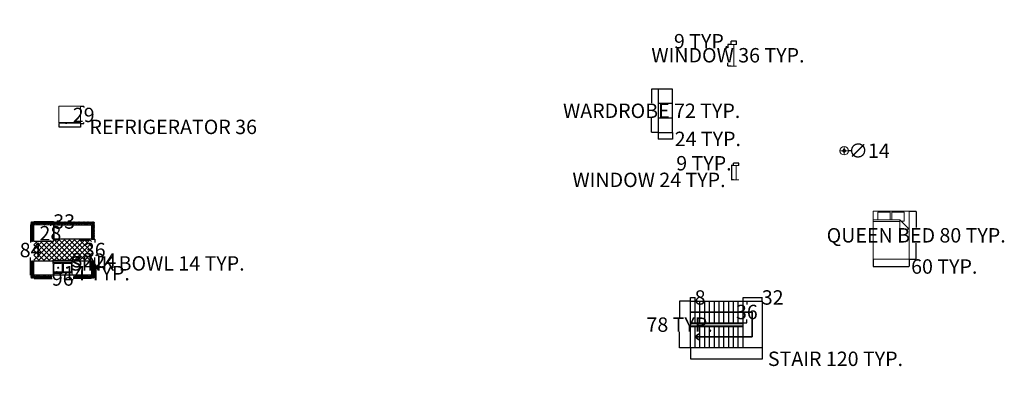
# Model space of a CAD drawing. Units: inches. Extents: x -1226 to 4538, y -998 to 1029.
# Tile 5 of 5: x 2895 to 4538, y 408 to 1029. Entities that reach past the tile are written whole.
import ezdxf

# ---------------------------------------------------------------- set-up
doc = ezdxf.new("R2010")
doc.units = ezdxf.units.IN
doc.header["$MEASUREMENT"] = 0
for name, color, linetype, lineweight in [('A-ANNO-DIMS', 2, 'Continuous', 18), ('A-ANNO-SYMB', 7, 'Continuous', 35), ('A-EQPM', 8, 'Continuous', 18), ('A-FLOR-CASE', 8, 'Continuous', 25), ('A-FLOR-FIXT', 9, 'Continuous', 18), ('A-FLOR-PATT', 2, 'Continuous', 13), ('A-FLOR-STRS', 7, 'Continuous', 25), ('A-FURN', 8, 'Continuous', 18), ('A-GLAZ', 3, 'Continuous', 18), ('A-WALL-PATT', 1, 'Continuous', 13)]:
    doc.layers.add(name, color=color, linetype=linetype, lineweight=lineweight)
doc.styles.get("Standard").update_dxf_attribs({"font": 'arial.ttf'})
doc.dimstyles.get("Standard").update_dxf_attribs({"dimtxt": 24, "dimasz": 0.18, "dimexe": 0.18, "dimexo": 0.0625, "dimgap": 0.09, "dimtad": 0, "dimtih": 1, "dimtoh": 1, "dimdec": 0, "dimzin": 0, "dimdsep": 46, "dimlunit": 4, "dimtxsty": 'Standard', "dimcen": 0.09, "dimadec": 0, "dimazin": 0, "dimtfac": 1, "dimtdec": 0, "dimtofl": 0, "dimtmove": 0, "dimatfit": 3, "dimfxl": 1, "dimtolj": 1, "dimtzin": 0, "dimarcsym": 0})

# ---------------------------------------------------------------- blocks, each defined once
blk = doc.blocks.new('Bed - Queen')
for p, q in [((0, -80.00003), (0, 0)), ((0, 0), (59.99999, 0)), ((59.99999, 0), (59.99999, -80.00003)), ((0, -14.4), (44.8, -14.4)), ((7.99999, -1.2), (28.79998, -1.2)), ((7.99999, -14.4), (7.99999, -1.2)), ((28.79998, -1.2), (28.79998, -14.4)), ((31.19999, -1.2), (51.99999, -1.2)), ((31.19999, -14.4), (31.19999, -1.2)), ((59.99999, -29.6), (44.8, -14.4)), ((44.8, -14.4), (44.8, -29.6)), ((51.99999, -16.4), (46.79936, -16.4)), ((51.99999, -1.2), (51.99999, -16.4)), ((44.8, -16.8), (0, -16.8)), ((44.8, -29.6), (59.99999, -29.6)), ((59.99999, -80.00003), (0, -80.00003))]:
    blk.add_line(p, q)
blk = doc.blocks.new('Lamp - Table')
for p, q in [((-1, 0), (-7, 0)), ((0, 3), (-3, 0)), ((-3, 0), (0, -3)), ((0, 7), (0, 1)), ((3, 0), (0, 3)), ((0, -3), (3, 0)), ((1, 0), (7, 0)), ((0, -1), (0, -7))]:
    blk.add_line(p, q)
for radius in [7, 1]:
    blk.add_circle((0, 0), radius)
blk = doc.blocks.new('Refrigerator-2 door - 36 in top')
for p, q in [((0, -26.999999), (36, -26.999999)), ((11, -27.999999), (11, -28.999999)), ((11, -28.999999), (13, -28.999999)), ((12, -26.999999), (12, -28.999999)), ((13, -28.999999), (13, -27.999999))]:
    blk.add_line(p, q)
blk.add_lwpolyline([(0, -27.999999), (0, 0), (36, 0), (36, -27.999999)], close=True)
blk = doc.blocks.new('WIN-36')
for p, q in [((0, 36), (9, 36)), ((4.5, 0), (4.5, 36)), ((0, 0), (9, 0))]:
    blk.add_line(p, q)
blk = doc.blocks.new('WIN-24')
for p, q in [((0, 24), (9, 24)), ((4.5, 0), (4.5, 24)), ((0, 0), (9, 0))]:
    blk.add_line(p, q)
blk = doc.blocks.new('WARDROBE-72X24')
for p, q in [((72, 24), (0, 24)), ((0, 24), (0, 0)), ((24, 24), (24, 0)), ((48, 24), (48, 0)), ((72, 0), (72, 24)), ((0, 0), (72, 0))]:
    blk.add_line(p, q)
blk = doc.blocks.new('STAIR-RETURN-120X78')
for p, q in [((0, 0), (0, 120)), ((0, 120), (78, 120)), ((78, 120), (78, 0)), ((42, 88), (0, 88)), ((36, 0), (36, 88)), ((37, 0), (37, 88)), ((41, 0), (41, 88)), ((42, 0), (42, 88)), ((78, 88), (42, 88)), ((36, 80), (0, 80)), ((36, 72), (0, 72)), ((78, 80), (42, 80)), ((78, 72), (42, 72)), ((36, 64), (0, 64)), ((36, 56), (0, 56)), ((78, 64), (42, 64)), ((78, 56), (42, 56)), ((36, 48), (0, 48)), ((36, 40), (0, 40)), ((78, 48), (42, 48)), ((78, 40), (42, 40)), ((36, 32), (0, 32)), ((36, 24), (0, 24)), ((78, 32), (42, 32)), ((78, 24), (42, 24)), ((36, 16), (0, 16)), ((36, 8), (0, 8)), ((78, 16), (42, 16)), ((78, 8), (42, 8)), ((37, 0), (0, 0)), ((78, 0), (41, 0))]:
    blk.add_line(p, q)
blk = doc.blocks.new('STAIR-DIRECTION-RETURN')
for p, q in [((0, 0), (0, 103.3)), ((0, 103.3), (40.8, 103.3)), ((40.8, 103.3), (40.8, 8)), ((40.8, 8), (35.9, 13.9)), ((40.8, 8), (45.7, 13.9))]:
    blk.add_line(p, q)
blk = doc.blocks.new('SINK-BOWL-COMPACT')
blk.add_line((13.8, 1), (13.8, 13))
for points in [[(0, 1), (0, 13)], [(1, 14), (12.8, 14)], [(12.8, 0), (1, 0)]]:
    blk.add_lwpolyline(points)
for radius in [1, 0.5]:
    blk.add_circle((7, 7), radius)
for centre, start, end in [((1, 13), 90, 180), ((1, 1), 180, 270), ((12.8, 13), 0, 90), ((12.8, 1), 270, 0)]:
    blk.add_arc(centre, 1, start, end)
blk = doc.blocks.new('*D22')
at = {"layer": 'A-ANNO-DIMS', "color": 0, "lineweight": -2, "transparency": 16777216}
for p, q in [((4082.1, 987.5), (4076.5, 987.5)), ((4076.7, 987.4), (4076.7, 982.1)), ((4076.7, 951.7), (4076.7, 957)), ((4082.1, 951.5), (4076.5, 951.5))]:
    blk.add_line(p, q, dxfattribs=at)
at = {"layer": 'A-ANNO-DIMS', "color": 0, "transparency": 16777216}
for points in [[(4076.7, 987.4), (4076.8, 987.4), (4076.7, 987.5)], [(4076.7, 951.7), (4076.8, 951.7), (4076.7, 951.5)]]:
    blk.add_solid(points, dxfattribs=at)
at = {"layer": 'Defpoints', "color": 0, "transparency": 16777216}
for p in [(4082.1, 987.5), (4076.7, 951.5), (4082.1, 951.5)]:
    blk.add_point(p, dxfattribs=at)
at = {"layer": 'A-ANNO-DIMS', "color": 0, "transparency": 16777216, "insert": (4076.7, 969.5), "char_height": 24, "attachment_point": 5}
blk.add_mtext('\\A1;WINDOW 36 TYP.', dxfattribs=at)
blk = doc.blocks.new('*D23')
at = {"layer": 'A-ANNO-DIMS', "color": 0, "lineweight": -2, "transparency": 16777216}
for p, q in [((4082.1, 992.9), (4081.9, 992.9)), ((4082.1, 987.6), (4082.1, 993.1)), ((4090.9, 992.9), (4082.3, 992.9)), ((4091.1, 987.6), (4091.1, 993.1))]:
    blk.add_line(p, q, dxfattribs=at)
at = {"layer": 'A-ANNO-DIMS', "color": 0, "transparency": 16777216}
for points in [[(4082.3, 993), (4082.3, 992.9), (4082.1, 992.9)], [(4090.9, 993), (4090.9, 992.9), (4091.1, 992.9)]]:
    blk.add_solid(points, dxfattribs=at)
at = {"layer": 'Defpoints', "color": 0, "transparency": 16777216}
for p in [(4082.1, 992.9), (4082.1, 987.5), (4091.1, 987.5)]:
    blk.add_point(p, dxfattribs=at)
at = {"layer": 'A-ANNO-DIMS', "color": 0, "transparency": 16777216, "insert": (4032.8, 992.9), "char_height": 24, "attachment_point": 5}
blk.add_mtext('\\A1;9 TYP.', dxfattribs=at)
blk = doc.blocks.new('*D24')
at = {"layer": 'A-ANNO-DIMS', "color": 0, "lineweight": -2, "transparency": 16777216}
for p, q in [((4086, 785.9), (4082.3, 785.9)), ((4082.5, 785.8), (4082.5, 762.1)), ((4086, 761.9), (4082.3, 761.9)), ((4082.5, 761.8), (4082.3, 761.8)), ((4082.5, 761.9), (4082.5, 761.8))]:
    blk.add_line(p, q, dxfattribs=at)
at = {"layer": 'A-ANNO-DIMS', "color": 0, "transparency": 16777216}
for points in [[(4082.4, 785.8), (4082.5, 785.8), (4082.5, 785.9)], [(4082.4, 762.1), (4082.5, 762.1), (4082.5, 761.9)]]:
    blk.add_solid(points, dxfattribs=at)
at = {"layer": 'Defpoints', "color": 0, "transparency": 16777216}
for p in [(4086.1, 785.9), (4082.5, 761.9), (4086.1, 761.9)]:
    blk.add_point(p, dxfattribs=at)
at = {"layer": 'A-ANNO-DIMS', "color": 0, "transparency": 16777216, "insert": (3945.1, 761.8), "char_height": 24, "attachment_point": 5}
blk.add_mtext('\\A1;WINDOW 24 TYP.', dxfattribs=at)
blk = doc.blocks.new('*D25')
at = {"layer": 'A-ANNO-DIMS', "color": 0, "lineweight": -2, "transparency": 16777216}
for p, q in [((4086.1, 789.5), (4085.9, 789.5)), ((4086.1, 786), (4086.1, 789.7)), ((4094.9, 789.5), (4086.2, 789.5)), ((4095.1, 786), (4095.1, 789.7))]:
    blk.add_line(p, q, dxfattribs=at)
at = {"layer": 'A-ANNO-DIMS', "color": 0, "transparency": 16777216}
for points in [[(4086.2, 789.6), (4086.2, 789.5), (4086.1, 789.5)], [(4094.9, 789.6), (4094.9, 789.5), (4095.1, 789.5)]]:
    blk.add_solid(points, dxfattribs=at)
at = {"layer": 'Defpoints', "color": 0, "transparency": 16777216}
for p in [(4086.1, 789.5), (4086.1, 785.9), (4095.1, 785.9)]:
    blk.add_point(p, dxfattribs=at)
at = {"layer": 'A-ANNO-DIMS', "color": 0, "transparency": 16777216, "insert": (4036.7, 789.5), "char_height": 24, "attachment_point": 5}
blk.add_mtext('\\A1;9 TYP.', dxfattribs=at)
blk = doc.blocks.new('*D30')
at = {"layer": 'A-ANNO-DIMS', "color": 0, "lineweight": -2, "transparency": 16777216}
for p, q in [((4378.9, 709.4), (4391, 709.4)), ((4390.8, 709.2), (4390.8, 682.6)), ((4390.8, 629.6), (4390.8, 656.2)), ((4378.9, 629.4), (4391, 629.4))]:
    blk.add_line(p, q, dxfattribs=at)
at = {"layer": 'A-ANNO-DIMS', "color": 0, "transparency": 16777216}
for points in [[(4390.8, 709.2), (4390.9, 709.2), (4390.8, 709.4)], [(4390.8, 629.6), (4390.9, 629.6), (4390.8, 629.4)]]:
    blk.add_solid(points, dxfattribs=at)
at = {"layer": 'Defpoints', "color": 0, "transparency": 16777216}
for p in [(4378.8, 709.4), (4390.8, 709.4), (4378.8, 629.4)]:
    blk.add_point(p, dxfattribs=at)
at = {"layer": 'A-ANNO-DIMS', "color": 0, "transparency": 16777216, "insert": (4390.8, 669.4), "char_height": 24, "attachment_point": 5}
blk.add_mtext('\\A1;QUEEN BED 80 TYP.', dxfattribs=at)
blk = doc.blocks.new('*D31')
at = {"layer": 'A-ANNO-DIMS', "color": 0, "lineweight": -2, "transparency": 16777216}
for p, q in [((4318.8, 629.3), (4318.8, 617.2)), ((4378.8, 629.3), (4378.8, 617.2)), ((4319, 617.4), (4378.7, 617.4)), ((4378.8, 617.4), (4379, 617.4))]:
    blk.add_line(p, q, dxfattribs=at)
at = {"layer": 'A-ANNO-DIMS', "color": 0, "transparency": 16777216}
for points in [[(4319, 617.4), (4319, 617.4), (4318.8, 617.4)], [(4378.7, 617.4), (4378.7, 617.4), (4378.8, 617.4)]]:
    blk.add_solid(points, dxfattribs=at)
at = {"layer": 'Defpoints', "color": 0, "transparency": 16777216}
for p in [(4318.8, 629.4), (4378.8, 629.4), (4378.8, 617.4)]:
    blk.add_point(p, dxfattribs=at)
at = {"layer": 'A-ANNO-DIMS', "color": 0, "transparency": 16777216, "insert": (4437.6, 617.4), "char_height": 24, "attachment_point": 5}
blk.add_mtext('\\A1;60 TYP.', dxfattribs=at)
blk = doc.blocks.new('*D32')
at = {"layer": 'A-ANNO-DIMS', "color": 0, "lineweight": -2, "transparency": 16777216}
for p, q in [((3960.3, 912.9), (3949.3, 912.9)), ((3949.5, 912.7), (3949.5, 889.4)), ((3949.5, 841.1), (3949.5, 864.4)), ((3960.3, 840.9), (3949.3, 840.9))]:
    blk.add_line(p, q, dxfattribs=at)
at = {"layer": 'A-ANNO-DIMS', "color": 0, "transparency": 16777216}
for points in [[(3949.5, 912.7), (3949.6, 912.7), (3949.5, 912.9)], [(3949.5, 841.1), (3949.6, 841.1), (3949.5, 840.9)]]:
    blk.add_solid(points, dxfattribs=at)
at = {"layer": 'Defpoints', "color": 0, "transparency": 16777216}
for p in [(3960.3, 912.9), (3949.5, 840.9), (3960.3, 840.9)]:
    blk.add_point(p, dxfattribs=at)
at = {"layer": 'A-ANNO-DIMS', "color": 0, "transparency": 16777216, "insert": (3949.5, 876.9), "char_height": 24, "attachment_point": 5}
blk.add_mtext('\\A1;WARDROBE 72 TYP.', dxfattribs=at)
blk = doc.blocks.new('*D33')
at = {"layer": 'A-ANNO-DIMS', "color": 0, "lineweight": -2, "transparency": 16777216}
for p, q in [((3960.3, 840.8), (3960.3, 829.9)), ((3984.3, 840.8), (3984.3, 829.9)), ((3960.5, 830.1), (3984.1, 830.1)), ((3984.3, 830.1), (3984.5, 830.1))]:
    blk.add_line(p, q, dxfattribs=at)
at = {"layer": 'A-ANNO-DIMS', "color": 0, "transparency": 16777216}
for points in [[(3960.5, 830.1), (3960.5, 830.1), (3960.3, 830.1)], [(3984.1, 830.1), (3984.1, 830.1), (3984.3, 830.1)]]:
    blk.add_solid(points, dxfattribs=at)
at = {"layer": 'Defpoints', "color": 0, "transparency": 16777216}
for p in [(3960.3, 840.9), (3984.3, 840.9), (3984.3, 830.1)]:
    blk.add_point(p, dxfattribs=at)
at = {"layer": 'A-ANNO-DIMS', "color": 0, "transparency": 16777216, "insert": (4043.2, 830.1), "char_height": 24, "attachment_point": 5}
blk.add_mtext('\\A1;24 TYP.', dxfattribs=at)
blk = doc.blocks.new('*D36')
at = {"layer": 'A-ANNO-DIMS', "color": 0, "lineweight": -2, "transparency": 16777216}
for p, q in [((4014.1, 481.5), (4014.1, 463.4)), ((4134.1, 481.5), (4134.1, 463.4)), ((4014.3, 463.6), (4133.9, 463.6)), ((4134.1, 463.6), (4134.3, 463.6))]:
    blk.add_line(p, q, dxfattribs=at)
at = {"layer": 'A-ANNO-DIMS', "color": 0, "transparency": 16777216}
for points in [[(4014.3, 463.6), (4014.3, 463.6), (4014.1, 463.6)], [(4133.9, 463.6), (4133.9, 463.6), (4134.1, 463.6)]]:
    blk.add_solid(points, dxfattribs=at)
at = {"layer": 'Defpoints', "color": 0, "transparency": 16777216}
for p in [(4014.1, 481.6), (4134.1, 481.6), (4134.1, 463.6)]:
    blk.add_point(p, dxfattribs=at)
at = {"layer": 'A-ANNO-DIMS', "color": 0, "transparency": 16777216, "insert": (4256.1, 463.6), "char_height": 24, "attachment_point": 5}
blk.add_mtext('\\A1;STAIR 120 TYP.', dxfattribs=at)
blk = doc.blocks.new('*D37')
at = {"layer": 'A-ANNO-DIMS', "color": 0, "lineweight": -2, "transparency": 16777216}
for p, q in [((4014, 559.6), (3995.9, 559.6)), ((3996.1, 559.4), (3996.1, 533)), ((3996.1, 481.8), (3996.1, 508.3)), ((4014, 481.6), (3995.9, 481.6))]:
    blk.add_line(p, q, dxfattribs=at)
at = {"layer": 'A-ANNO-DIMS', "color": 0, "transparency": 16777216}
for points in [[(3996.1, 559.4), (3996.1, 559.4), (3996.1, 559.6)], [(3996.1, 481.8), (3996.1, 481.8), (3996.1, 481.6)]]:
    blk.add_solid(points, dxfattribs=at)
at = {"layer": 'Defpoints', "color": 0, "transparency": 16777216}
for p in [(4014.1, 559.6), (3996.1, 481.6), (4014.1, 481.6)]:
    blk.add_point(p, dxfattribs=at)
at = {"layer": 'A-ANNO-DIMS', "color": 0, "transparency": 16777216, "insert": (3996.1, 520.6), "char_height": 24, "attachment_point": 5}
blk.add_mtext('\\A1;78 TYP.', dxfattribs=at)
blk = doc.blocks.new('*D38')
at = {"layer": 'A-ANNO-DIMS', "color": 0, "lineweight": -2, "transparency": 16777216}
for p, q in [((2966.3, 622.4), (2968.5, 622.4)), ((2966.3, 608.4), (2968.5, 608.4)), ((2968.3, 622.4), (2968.3, 622.6)), ((2968.3, 622.6), (2968.5, 622.6)), ((2968.3, 608.6), (2968.3, 622.2))]:
    blk.add_line(p, q, dxfattribs=at)
at = {"layer": 'A-ANNO-DIMS', "color": 0, "transparency": 16777216}
for points in [[(2968.3, 622.2), (2968.4, 622.2), (2968.3, 622.4)], [(2968.3, 608.6), (2968.4, 608.6), (2968.3, 608.4)]]:
    blk.add_solid(points, dxfattribs=at)
at = {"layer": 'Defpoints', "color": 0, "transparency": 16777216}
for p in [(2966.2, 622.4), (2966.2, 608.4), (2968.3, 622.4)]:
    blk.add_point(p, dxfattribs=at)
at = {"layer": 'A-ANNO-DIMS', "color": 0, "transparency": 16777216, "insert": (3124.8, 622.6), "char_height": 24, "attachment_point": 5}
blk.add_mtext('\\A1;SINK BOWL 14 TYP.', dxfattribs=at)
blk = doc.blocks.new('*D39')
at = {"layer": 'A-ANNO-DIMS', "color": 0, "lineweight": -2, "transparency": 16777216}
for p, q in [((2952.5, 608.3), (2952.5, 606.1)), ((2966.2, 608.3), (2966.2, 606.1)), ((2952.7, 606.3), (2966.1, 606.3)), ((2966.2, 606.3), (2966.4, 606.3))]:
    blk.add_line(p, q, dxfattribs=at)
at = {"layer": 'A-ANNO-DIMS', "color": 0, "transparency": 16777216}
for points in [[(2952.7, 606.3), (2952.7, 606.2), (2952.5, 606.3)], [(2966.1, 606.3), (2966.1, 606.2), (2966.2, 606.3)]]:
    blk.add_solid(points, dxfattribs=at)
at = {"layer": 'Defpoints', "color": 0, "transparency": 16777216}
for p in [(2952.5, 608.4), (2966.2, 608.4), (2966.2, 606.3)]:
    blk.add_point(p, dxfattribs=at)
at = {"layer": 'A-ANNO-DIMS', "color": 0, "transparency": 16777216, "insert": (3023.8, 606.3), "char_height": 24, "attachment_point": 5}
blk.add_mtext('\\A1;14 TYP.', dxfattribs=at)
blk = doc.blocks.new('*D42')
at = {"layer": 'A-ANNO-DIMS', "color": 0, "lineweight": -2, "transparency": 16777216}
for p, q in [((2960.7, 855.4), (2960.7, 849.9)), ((2996.7, 855.4), (2996.7, 849.9)), ((2960.9, 850.1), (2996.5, 850.1)), ((2996.7, 850.1), (2996.9, 850.1))]:
    blk.add_line(p, q, dxfattribs=at)
at = {"layer": 'A-ANNO-DIMS', "color": 0, "transparency": 16777216}
for points in [[(2960.9, 850.1), (2960.9, 850), (2960.7, 850.1)], [(2996.5, 850.1), (2996.5, 850), (2996.7, 850.1)]]:
    blk.add_solid(points, dxfattribs=at)
at = {"layer": 'Defpoints', "color": 0, "transparency": 16777216}
for p in [(2960.7, 855.5), (2996.7, 855.5), (2996.7, 850.1)]:
    blk.add_point(p, dxfattribs=at)
at = {"layer": 'A-ANNO-DIMS', "color": 0, "transparency": 16777216, "insert": (3151.4, 850.1), "char_height": 24, "attachment_point": 5}
blk.add_mtext('\\A1;REFRIGERATOR 36', dxfattribs=at)
blk = doc.blocks.new('*D43')
at = {"layer": 'A-ANNO-DIMS', "color": 0, "lineweight": -2, "transparency": 16777216}
for p, q in [((2996.8, 884.5), (3002.3, 884.5)), ((3002.1, 884.3), (3002.1, 882.3)), ((2996.8, 855.5), (3002.3, 855.5)), ((3002.1, 855.7), (3002.1, 857.6))]:
    blk.add_line(p, q, dxfattribs=at)
at = {"layer": 'A-ANNO-DIMS', "color": 0, "transparency": 16777216}
for points in [[(3002.1, 884.3), (3002.1, 884.3), (3002.1, 884.5)], [(3002.1, 855.7), (3002.1, 855.7), (3002.1, 855.5)]]:
    blk.add_solid(points, dxfattribs=at)
at = {"layer": 'Defpoints', "color": 0, "transparency": 16777216}
for p in [(2996.7, 884.5), (3002.1, 884.5), (2996.7, 855.5)]:
    blk.add_point(p, dxfattribs=at)
at = {"layer": 'A-ANNO-DIMS', "color": 0, "transparency": 16777216, "insert": (3002.1, 870), "char_height": 24, "attachment_point": 5}
blk.add_mtext('\\A1;29', dxfattribs=at)
blk = doc.blocks.new('*D67')
at = {"layer": 'A-ANNO-DIMS', "color": 0, "lineweight": -2, "transparency": 16777216}
for p, q in [((2919, 602.8), (2919, 597.2)), ((2919.2, 597.4), (2949.7, 597.4)), ((3014.8, 597.4), (2984.3, 597.4)), ((3015, 602.8), (3015, 597.2))]:
    blk.add_line(p, q, dxfattribs=at)
at = {"layer": 'A-ANNO-DIMS', "color": 0, "transparency": 16777216}
for points in [[(2919.2, 597.4), (2919.2, 597.3), (2919, 597.4)], [(3014.8, 597.4), (3014.8, 597.3), (3015, 597.4)]]:
    blk.add_solid(points, dxfattribs=at)
at = {"layer": 'Defpoints', "color": 0, "transparency": 16777216}
for p in [(2919, 602.9), (3015, 602.9), (3015, 597.4)]:
    blk.add_point(p, dxfattribs=at)
at = {"layer": 'A-ANNO-DIMS', "color": 0, "transparency": 16777216, "insert": (2967, 597.4), "char_height": 24, "attachment_point": 5}
blk.add_mtext('\\A1;96', dxfattribs=at)
blk = doc.blocks.new('*D68')
at = {"layer": 'A-ANNO-DIMS', "color": 0, "lineweight": -2, "transparency": 16777216}
for p, q in [((2918.9, 686.9), (2913.3, 686.9)), ((2913.5, 686.7), (2913.5, 657.2)), ((2913.5, 603.1), (2913.5, 632.5)), ((2918.9, 602.9), (2913.3, 602.9))]:
    blk.add_line(p, q, dxfattribs=at)
at = {"layer": 'A-ANNO-DIMS', "color": 0, "transparency": 16777216}
for points in [[(2913.5, 686.7), (2913.5, 686.7), (2913.5, 686.9)], [(2913.5, 603.1), (2913.5, 603.1), (2913.5, 602.9)]]:
    blk.add_solid(points, dxfattribs=at)
at = {"layer": 'Defpoints', "color": 0, "transparency": 16777216}
for p in [(2919, 686.9), (2913.5, 602.9), (2919, 602.9)]:
    blk.add_point(p, dxfattribs=at)
at = {"layer": 'A-ANNO-DIMS', "color": 0, "transparency": 16777216, "insert": (2913.5, 644.9), "char_height": 24, "attachment_point": 5}
blk.add_mtext('\\A1;84', dxfattribs=at)
blk = doc.blocks.new('*D69')
at = {"layer": 'A-ANNO-DIMS', "color": 0, "lineweight": -2, "transparency": 16777216}
for p, q in [((3015, 626.9), (3020.7, 626.9)), ((3020.5, 626.9), (3020.5, 627.1)), ((3020.5, 627.1), (3020.7, 627.1)), ((3020.5, 603.1), (3020.5, 626.7)), ((3015, 602.9), (3020.7, 602.9))]:
    blk.add_line(p, q, dxfattribs=at)
at = {"layer": 'A-ANNO-DIMS', "color": 0, "transparency": 16777216}
for points in [[(3020.5, 626.7), (3020.5, 626.7), (3020.5, 626.9)], [(3020.5, 603.1), (3020.5, 603.1), (3020.5, 602.9)]]:
    blk.add_solid(points, dxfattribs=at)
at = {"layer": 'Defpoints', "color": 0, "transparency": 16777216}
for p in [(3015, 626.9), (3020.5, 626.9), (3015, 602.9)]:
    blk.add_point(p, dxfattribs=at)
at = {"layer": 'A-ANNO-DIMS', "color": 0, "transparency": 16777216, "insert": (3038.1, 627.1), "char_height": 24, "attachment_point": 5}
blk.add_mtext('\\A1;24', dxfattribs=at)
blk = doc.blocks.new('*D70')
at = {"layer": 'A-ANNO-DIMS', "color": 0, "lineweight": -2, "transparency": 16777216}
for p, q in [((3015, 662.9), (3020.7, 662.9)), ((3020.5, 662.7), (3020.5, 657.2)), ((3015, 626.9), (3020.7, 626.9)), ((3020.5, 627.1), (3020.5, 632.5))]:
    blk.add_line(p, q, dxfattribs=at)
at = {"layer": 'A-ANNO-DIMS', "color": 0, "transparency": 16777216}
for points in [[(3020.5, 662.7), (3020.5, 662.7), (3020.5, 662.9)], [(3020.5, 627.1), (3020.5, 627.1), (3020.5, 626.9)]]:
    blk.add_solid(points, dxfattribs=at)
at = {"layer": 'Defpoints', "color": 0, "transparency": 16777216}
for p in [(3015, 662.9), (3020.5, 662.9), (3015, 626.9)]:
    blk.add_point(p, dxfattribs=at)
at = {"layer": 'A-ANNO-DIMS', "color": 0, "transparency": 16777216, "insert": (3020.5, 644.9), "char_height": 24, "attachment_point": 5}
blk.add_mtext('\\A1;36', dxfattribs=at)
blk = doc.blocks.new('*D71')
at = {"layer": 'A-ANNO-DIMS', "color": 0, "lineweight": -2, "transparency": 16777216}
for p, q in [((2919, 686.9), (2919, 692.6)), ((2919.2, 692.4), (2951.8, 692.4)), ((2952, 686.9), (2952, 692.6)), ((2952, 692.4), (2952.2, 692.4))]:
    blk.add_line(p, q, dxfattribs=at)
at = {"layer": 'A-ANNO-DIMS', "color": 0, "transparency": 16777216}
for points in [[(2919.2, 692.4), (2919.2, 692.3), (2919, 692.4)], [(2951.8, 692.4), (2951.8, 692.3), (2952, 692.4)]]:
    blk.add_solid(points, dxfattribs=at)
at = {"layer": 'Defpoints', "color": 0, "transparency": 16777216}
for p in [(2952, 692.4), (2919, 686.9), (2952, 686.9)]:
    blk.add_point(p, dxfattribs=at)
at = {"layer": 'A-ANNO-DIMS', "color": 0, "transparency": 16777216, "insert": (2969.4, 692.4), "char_height": 24, "attachment_point": 5}
blk.add_mtext('\\A1;33', dxfattribs=at)
blk = doc.blocks.new('*D72')
at = {"layer": 'A-ANNO-DIMS', "color": 0, "lineweight": -2, "transparency": 16777216}
for p, q in [((2951.9, 686.9), (2946.3, 686.9)), ((2946.5, 686.7), (2946.5, 685.2)), ((2951.9, 658.9), (2946.3, 658.9)), ((2946.5, 659.1), (2946.5, 660.5))]:
    blk.add_line(p, q, dxfattribs=at)
at = {"layer": 'A-ANNO-DIMS', "color": 0, "transparency": 16777216}
for points in [[(2946.5, 686.7), (2946.5, 686.7), (2946.5, 686.9)], [(2946.5, 659.1), (2946.5, 659.1), (2946.5, 658.9)]]:
    blk.add_solid(points, dxfattribs=at)
at = {"layer": 'Defpoints', "color": 0, "transparency": 16777216}
for p in [(2946.5, 686.9), (2952, 686.9), (2952, 658.9)]:
    blk.add_point(p, dxfattribs=at)
at = {"layer": 'A-ANNO-DIMS', "color": 0, "transparency": 16777216, "insert": (2946.5, 672.9), "char_height": 24, "attachment_point": 5}
blk.add_mtext('\\A1;28', dxfattribs=at)
blk = doc.blocks.new('*D73')
at = {"layer": 'A-ANNO-DIMS', "color": 0, "lineweight": -2, "transparency": 16777216}
for p, q in [((2951, 622.4), (2951, 628.1)), ((2951.2, 627.9), (2982.8, 627.9)), ((2983, 622.4), (2983, 628.1)), ((2983, 627.9), (2983.2, 627.9))]:
    blk.add_line(p, q, dxfattribs=at)
at = {"layer": 'A-ANNO-DIMS', "color": 0, "transparency": 16777216}
for points in [[(2951.2, 627.9), (2951.2, 627.8), (2951, 627.9)], [(2982.8, 627.9), (2982.8, 627.8), (2983, 627.9)]]:
    blk.add_solid(points, dxfattribs=at)
at = {"layer": 'Defpoints', "color": 0, "transparency": 16777216}
for p in [(2983, 627.9), (2951, 622.4), (2983, 622.4)]:
    blk.add_point(p, dxfattribs=at)
at = {"layer": 'A-ANNO-DIMS', "color": 0, "transparency": 16777216, "insert": (3000.3, 627.9), "char_height": 24, "attachment_point": 5}
blk.add_mtext('\\A1;32', dxfattribs=at)
blk = doc.blocks.new('*D74')
at = {"layer": 'A-ANNO-DIMS', "color": 0, "lineweight": -2, "transparency": 16777216}
for p, q in [((4014.1, 559.7), (4014.1, 566)), ((4014.3, 565.8), (4021.9, 565.8)), ((4022.1, 559.7), (4022.1, 566)), ((4022.1, 565.8), (4022.3, 565.8))]:
    blk.add_line(p, q, dxfattribs=at)
at = {"layer": 'A-ANNO-DIMS', "color": 0, "transparency": 16777216}
for points in [[(4014.3, 565.8), (4014.3, 565.8), (4014.1, 565.8)], [(4021.9, 565.8), (4021.9, 565.8), (4022.1, 565.8)]]:
    blk.add_solid(points, dxfattribs=at)
at = {"layer": 'Defpoints', "color": 0, "transparency": 16777216}
for p in [(4014.1, 559.6), (4022.1, 565.8), (4022.1, 559.6)]:
    blk.add_point(p, dxfattribs=at)
at = {"layer": 'A-ANNO-DIMS', "color": 0, "transparency": 16777216, "insert": (4030.3, 565.8), "char_height": 24, "attachment_point": 5}
blk.add_mtext('\\A1;8', dxfattribs=at)
blk = doc.blocks.new('*D75')
at = {"layer": 'A-ANNO-DIMS', "color": 0, "lineweight": -2, "transparency": 16777216}
for p, q in [((4102.1, 559.7), (4102.1, 566)), ((4102.3, 565.8), (4133.9, 565.8)), ((4134.1, 559.7), (4134.1, 566)), ((4134.1, 565.8), (4134.3, 565.8))]:
    blk.add_line(p, q, dxfattribs=at)
at = {"layer": 'A-ANNO-DIMS', "color": 0, "transparency": 16777216}
for points in [[(4102.3, 565.8), (4102.3, 565.8), (4102.1, 565.8)], [(4133.9, 565.8), (4133.9, 565.8), (4134.1, 565.8)]]:
    blk.add_solid(points, dxfattribs=at)
at = {"layer": 'Defpoints', "color": 0, "transparency": 16777216}
for p in [(4102.1, 559.6), (4134.1, 565.8), (4134.1, 559.6)]:
    blk.add_point(p, dxfattribs=at)
at = {"layer": 'A-ANNO-DIMS', "color": 0, "transparency": 16777216, "insert": (4151.4, 565.8), "char_height": 24, "attachment_point": 5}
blk.add_mtext('\\A1;32', dxfattribs=at)
blk = doc.blocks.new('*D76')
at = {"layer": 'A-ANNO-DIMS', "color": 0, "lineweight": -2, "transparency": 16777216}
for p, q in [((4102.1, 559.6), (4108.5, 559.6)), ((4108.3, 559.4), (4108.3, 554)), ((4108.3, 523.8), (4108.3, 529.3)), ((4102.1, 523.6), (4108.5, 523.6))]:
    blk.add_line(p, q, dxfattribs=at)
at = {"layer": 'A-ANNO-DIMS', "color": 0, "transparency": 16777216}
for points in [[(4108.3, 559.4), (4108.3, 559.4), (4108.3, 559.6)], [(4108.3, 523.8), (4108.3, 523.8), (4108.3, 523.6)]]:
    blk.add_solid(points, dxfattribs=at)
at = {"layer": 'Defpoints', "color": 0, "transparency": 16777216}
for p in [(4102.1, 559.6), (4102.1, 523.6), (4108.3, 523.6)]:
    blk.add_point(p, dxfattribs=at)
at = {"layer": 'A-ANNO-DIMS', "color": 0, "transparency": 16777216, "insert": (4108.3, 541.6), "char_height": 24, "attachment_point": 5}
blk.add_mtext('\\A1;36', dxfattribs=at)
blk = doc.blocks.new('*D83')
at = {"layer": 'A-ANNO-DIMS', "color": 0, "lineweight": -2, "transparency": 16777216}
for p, q in [((4270.5, 810.4), (4270.7, 810.4)), ((4270.6, 810.3), (4270.6, 810.5)), ((4281.8, 810.4), (4277.8, 810.4))]:
    blk.add_line(p, q, dxfattribs=at)
at = {"layer": 'A-ANNO-DIMS', "color": 0, "transparency": 16777216}
blk.add_solid([(4277.8, 810.4), (4277.8, 810.3), (4277.6, 810.4)], dxfattribs=at)
at = {"layer": 'Defpoints', "color": 0, "transparency": 16777216}
for p in [(4263.6, 810.4), (4277.6, 810.4)]:
    blk.add_point(p, dxfattribs=at)
at = {"layer": 'A-ANNO-DIMS', "color": 0, "transparency": 16777216, "insert": (4312.1, 810.4), "char_height": 24, "attachment_point": 5}
blk.add_mtext('\\A1;∅14', dxfattribs=at)

msp = doc.modelspace()

# ---------------------------------------------------------------- hatches: boundary and pattern name
at = {"layer": 'A-FLOR-PATT'}
h = msp.add_hatch(dxfattribs=at)
h.set_pattern_fill('ANSI37', color=256, scale=48, style=0)
h.paths.add_polyline_path([(2918.9813, 626.8792), (3014.9813, 626.8792), (3014.9813, 662.3792), (3012.9813, 662.3792), (3012.5413, 660.3792), (2994.4213, 660.3792), (2993.9813, 662.3792), (2952.9813, 662.3792), (2951.9813, 657.8791), (2918.9813, 657.8791)])
at = {"layer": 'A-WALL-PATT'}
h = msp.add_hatch(dxfattribs=at)
h.set_pattern_fill('ANSI37', color=256, scale=12, style=0)
h.paths.add_polyline_path([(2913.9813, 658.8792), (2917.9813, 658.8792), (2917.9813, 687.8792), (3015.9813, 687.8792), (3015.9813, 662.8792), (3019.9813, 662.8792), (3019.9813, 691.8792), (2913.9813, 691.8792)])
h = msp.add_hatch(dxfattribs=at)
h.set_pattern_fill('ANSI37', color=256, scale=12, style=0)
h.paths.add_polyline_path([(2913.9813, 597.8792), (2948.9813, 597.8792), (2948.9813, 601.8792), (2917.9813, 601.8792), (2917.9813, 626.8792), (2913.9813, 626.8792)])
h = msp.add_hatch(dxfattribs=at)
h.set_pattern_fill('ANSI37', color=256, scale=12, style=0)
h.paths.add_polyline_path([(2984.9813, 597.8792), (3019.9813, 597.8792), (3019.9813, 626.8792), (3015.9813, 626.8792), (3015.9813, 601.8792), (2984.9813, 601.8792)])

# ---------------------------------------------------------------- linework, layer by layer
at = {"layer": 'A-EQPM'}
for p, q in [((2918.9813, 659.8791), (2951.9813, 659.8791)), ((2949.9813, 657.8791), (2949.9813, 658.8791)), ((2950.9813, 657.8791), (2949.9813, 657.8791)), ((2950.9813, 658.8791), (2950.9813, 657.8791)), ((2998.9813, 662.8792), (2998.9813, 661.8792)), ((3000.9813, 661.8792), (3000.9813, 662.8792)), ((3005.9813, 661.8792), (3005.9813, 662.8792)), ((3007.9813, 662.8792), (3007.9813, 661.8792))]:
    msp.add_line(p, q, dxfattribs=at)
for points in [[(2918.9813, 658.8791), (2918.9813, 686.8792), (2951.9813, 686.8792), (2951.9813, 658.8791)], [(2994.9813, 660.8792), (2994.9813, 661.8792), (3011.9813, 661.8792), (3011.9813, 660.8792)]]:
    msp.add_lwpolyline(points, close=True, dxfattribs=at)
at = {"layer": 'A-FLOR-CASE'}
for p, q in [((2952.9813, 686.8792), (3014.9813, 686.8792)), ((2952.9813, 662.8792), (2952.9813, 686.8792)), ((3014.9813, 686.8792), (3014.9813, 662.8792)), ((3014.9813, 662.8792), (2952.9813, 662.8792)), ((2918.9813, 626.8792), (3014.9813, 626.8792)), ((2918.9813, 602.8792), (2918.9813, 626.8792)), ((3014.9813, 626.8792), (3014.9813, 602.8792)), ((3014.9813, 602.8792), (2918.9813, 602.8792))]:
    msp.add_line(p, q, dxfattribs=at)
at = {"layer": 'A-FLOR-FIXT'}
msp.add_line((2982.9813, 606.8792), (2950.9813, 606.8792), dxfattribs=at)
for points in [[(2950.9813, 604.3792), (2950.9813, 622.3792)], [(2952.4813, 623.8792), (2981.4813, 623.8792)], [(2982.9813, 622.3792), (2982.9813, 604.3792)], [(2981.4813, 602.8792), (2952.4813, 602.8792)]]:
    msp.add_lwpolyline(points, dxfattribs=at)
for centre, start, end in [((2952.4813, 622.3792), 90, 180), ((2981.4813, 622.3792), 0, 90), ((2952.4813, 604.3792), 180, 270), ((2981.4813, 604.3792), 270, 0)]:
    msp.add_arc(centre, 1.5, start, end, dxfattribs=at)

# ---------------------------------------------------------------- block references
at = {"layer": 'A-ANNO-SYMB', "rotation": 270.0000000000005}
msp.add_blockref('STAIR-DIRECTION-RETURN', (4014.0829, 541.108), dxfattribs=at)
at = {"layer": 'A-EQPM'}
msp.add_blockref('Refrigerator-2 door - 36 in top', (2960.699, 884.4782), dxfattribs=at)
at = {"layer": 'A-FLOR-CASE', "rotation": 269.9999999999993}
msp.add_blockref('WARDROBE-72X24', (3960.3294, 912.8834), dxfattribs=at)
at = {"layer": 'A-FLOR-FIXT'}
msp.add_blockref('SINK-BOWL-COMPACT', (2952.481, 608.379), dxfattribs=at)
at = {"layer": 'A-FLOR-FIXT', "rotation": 180}
msp.add_blockref('SINK-BOWL-COMPACT', (2981.4816, 622.3794), dxfattribs=at)
at = {"layer": 'A-FLOR-STRS', "rotation": 270.0000000000004}
msp.add_blockref('STAIR-RETURN-120X78', (4014.0829, 559.608), dxfattribs=at)
at = {"layer": 'A-FURN'}
for name, p in [('Lamp - Table', (4270.6338, 810.3732)), ('Bed - Queen', (4318.8409, 709.4051))]:
    msp.add_blockref(name, p, dxfattribs=at)
at = {"layer": 'A-GLAZ', "rotation": 180}
for name, p in [('WIN-36', (4091.1221, 987.5369)), ('WIN-24', (4095.0602, 785.9484))]:
    msp.add_blockref(name, p, dxfattribs=at)

# ---------------------------------------------------------------- dimensions: what is measured, and where the dimension line sits
at = {"layer": 'A-ANNO-DIMS'}
for base, p1, p2, angle, text, picture, middle in [((4076.7221, 951.5373), (4082.1221, 987.5373), (4082.1221, 951.5373), 270, 'WINDOW <> TYP.', '*D22', (4076.7221, 969.5373)), ((4082.1221, 992.9373), (4091.1221, 987.5373), (4082.1221, 987.5373), 180, '<> TYP.', '*D23', (4032.7635, 992.9373)), ((3949.5293, 840.8837), (3960.3293, 912.8837), (3960.3293, 840.8837), 270, 'WARDROBE <> TYP.', '*D32', (3949.5293, 876.8837)), ((4086.0605, 789.5483), (4095.0605, 785.9483), (4086.0605, 785.9483), 180, '<> TYP.', '*D25', (4036.7019, 789.5483)), ((4082.4605, 761.9483), (4086.0605, 785.9483), (4086.0605, 761.9483), 270, 'WINDOW <> TYP.', '*D24', (3945.0746, 761.7683)), ((4390.8409, 709.4051), (4378.8409, 629.4051), (4378.8409, 709.4051), 90, 'QUEEN BED <> TYP.', '*D30', (4390.8409, 669.4051)), ((2968.3313, 622.3792), (2966.2313, 608.3792), (2966.2313, 622.3792), 90, 'SINK BOWL <> TYP.', '*D38', (3124.765, 622.5592)), ((3996.0824, 481.6081), (4014.0824, 559.6081), (4014.0824, 481.6081), 270, '<> TYP.', '*D37', (3996.0824, 520.6081)), ((4134.0824, 463.6081), (4014.0824, 481.6081), (4134.0824, 481.6081), 0, 'STAIR <> TYP.', '*D36', (4256.055, 463.6081))]:
    dim = msp.add_linear_dim(base=base, p1=p1, p2=p2, angle=angle, text=text, dimstyle='Standard', override={"dimdec": 0, "dimlfac": 1, "dimrnd": 0, "dimzin": 0, "dimdsep": 46, "dimlunit": 2}, dxfattribs=at)
    dim.commit()
    dim.dimension.update_dxf_attribs({"geometry": picture, "text_midpoint": middle})
for base, p1, p2, text, picture, middle in [((2996.699, 850.0782), (2960.699, 855.4782), (2996.699, 855.4782), 'REFRIGERATOR <>', '*D42', (3151.3728, 850.0782)), ((3984.3293, 830.0837), (3960.3293, 840.8837), (3984.3293, 840.8837), '<> TYP.', '*D33', (4043.216, 830.0837)), ((2966.2313, 606.2792), (2952.4813, 608.3792), (2966.2313, 608.3792), '<> TYP.', '*D39', (3023.7837, 606.2792)), ((4378.8409, 617.4051), (4318.8409, 629.4051), (4378.8409, 629.4051), '<> TYP.', '*D31', (4437.5884, 617.4051))]:
    dim = msp.add_linear_dim(base=base, p1=p1, p2=p2, text=text, dimstyle='Standard', override={"dimdec": 0, "dimlfac": 1, "dimrnd": 0, "dimzin": 0, "dimdsep": 46, "dimlunit": 2}, dxfattribs=at)
    dim.commit()
    dim.dimension.update_dxf_attribs({"geometry": picture, "text_midpoint": middle})
for base, p1, p2, angle, picture, middle in [((3002.099, 884.4782), (2996.699, 855.4782), (2996.699, 884.4782), 90, '*D43', (3002.099, 869.9782)), ((2913.4813, 602.8792), (2918.9813, 686.8792), (2918.9813, 602.8792), 90, '*D68', (2913.4813, 644.8792)), ((2946.4813, 686.8792), (2951.9813, 658.8791), (2951.9813, 686.8792), 90, '*D72', (2946.4813, 672.8792)), ((3020.4813, 662.8792), (3014.9813, 626.8792), (3014.9813, 662.8792), 90, '*D70', (3020.4813, 644.8792)), ((3020.4813, 626.8792), (3014.9813, 602.8792), (3014.9813, 626.8792), 90, '*D69', (3038.0965, 627.0592)), ((4108.2824, 523.6081), (4102.0824, 559.6081), (4102.0824, 523.6081), 270, '*D76', (4108.2824, 541.6081))]:
    dim = msp.add_linear_dim(base=base, p1=p1, p2=p2, angle=angle, dimstyle='Standard', override={"dimdec": 0, "dimlfac": 1, "dimrnd": 0, "dimzin": 0, "dimdsep": 46, "dimlunit": 2}, dxfattribs=at)
    dim.commit()
    dim.dimension.update_dxf_attribs({"geometry": picture, "text_midpoint": middle})
dim = msp.add_diameter_dim_2p(p1=(4263.6338, 810.3734), p2=(4277.6338, 810.373), dimstyle='Standard', override={"dimdec": 0, "dimlfac": 1, "dimrnd": 0, "dimzin": 0, "dimdsep": 46, "dimlunit": 2}, dxfattribs=at)
dim.commit()
dim.dimension.update_dxf_attribs({"geometry": '*D83', "text_midpoint": (4281.8338, 810.3729), "dimtype": 163})
for base, p1, p2, picture, middle in [((2951.9813, 692.3792), (2918.9813, 686.8792), (2951.9813, 686.8792), '*D71', (2969.4327, 692.3792)), ((2982.9813, 627.8792), (2950.9813, 622.3792), (2982.9813, 622.3792), '*D73', (3000.31, 627.8792)), ((3014.9813, 597.3792), (2918.9813, 602.8792), (3014.9813, 602.8792), '*D67', (2966.9813, 597.3792)), ((4022.0824, 565.8081), (4014.0824, 559.6081), (4022.0824, 559.6081), '*D74', (4030.2596, 565.8081)), ((4134.0824, 565.8081), (4102.0824, 559.6081), (4134.0824, 559.6081), '*D75', (4151.4111, 565.8081))]:
    dim = msp.add_linear_dim(base=base, p1=p1, p2=p2, dimstyle='Standard', override={"dimdec": 0, "dimlfac": 1, "dimrnd": 0, "dimzin": 0, "dimdsep": 46, "dimlunit": 2}, dxfattribs=at)
    dim.commit()
    dim.dimension.update_dxf_attribs({"geometry": picture, "text_midpoint": middle})

doc.saveas('drawing.dxf')
